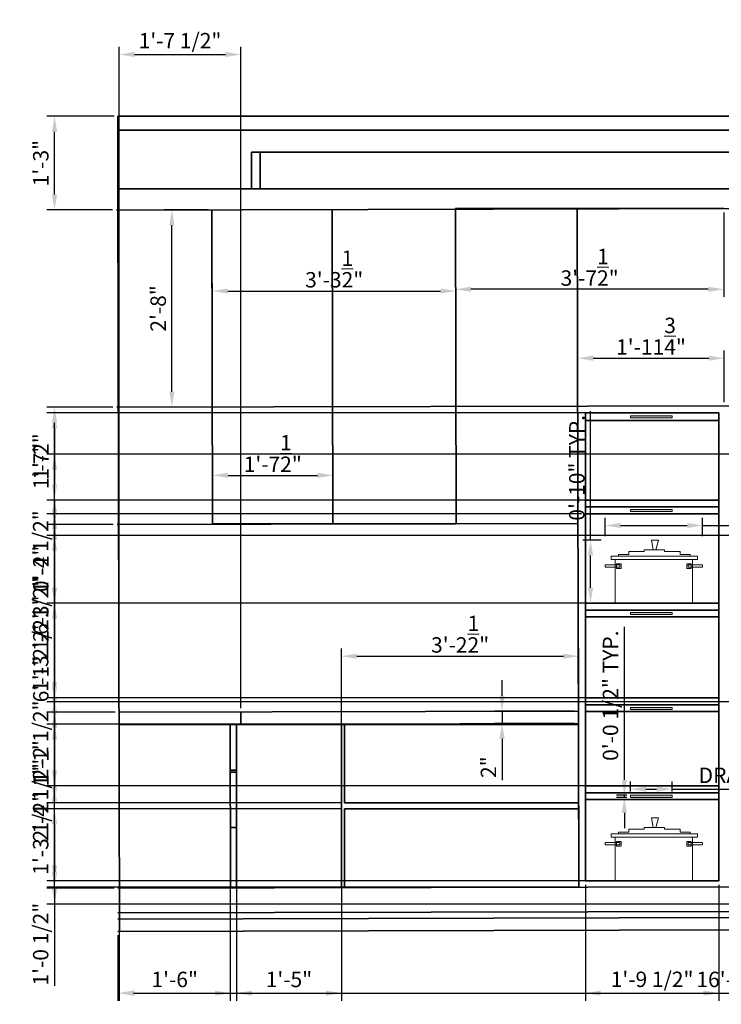
# Model space of a CAD drawing. Units: inches. Extents: x 1464 to 1689, y 996 to 1156.
# Tile 1 of 2: x 1464 to 1578, y 996 to 1156. Entities that reach past the tile are written whole.
import ezdxf

# ---------------------------------------------------------------- set-up
doc = ezdxf.new("R2010")
doc.units = ezdxf.units.IN
for name, color, linetype, lineweight in [('A-ANNO-DIMS', 2, 'Continuous', 18), ('A-ELEV', 7, 'Continuous', 35), ('A-EQPM', 9, 'Continuous', 18), ('A-FURN', 8, 'Continuous', 18)]:
    doc.layers.add(name, color=color, linetype=linetype, lineweight=lineweight)
doc.styles.get("Standard").update_dxf_attribs({"font": 'arial.ttf'})
doc.dimstyles.new('ISO-25', dxfattribs={"dimtxt": 2.5, "dimasz": 2.5, "dimexe": 1.25, "dimexo": 0.625, "dimtad": 1, "dimdec": 4, "dimlunit": 4, "dimtxsty": 'Standard', "dimcen": 2.5, "dimadec": 0, "dimazin": 0, "dimtfac": 1, "dimtdec": 4, "dimtmove": 0, "dimatfit": 3, "dimfxl": 1, "dimarcsym": 0})

# ---------------------------------------------------------------- blocks, each defined once
blk = doc.blocks.new('*D1')
at = {"layer": 'A-ANNO-DIMS', "color": 0, "lineweight": -2, "transparency": 16777216}
for p, q in [((1494.58, 1125.08), (1487.46, 1125.08)), ((1488.71, 1095.58), (1488.71, 1122.58)), ((1494.65, 1093.08), (1487.46, 1093.08))]:
    blk.add_line(p, q, dxfattribs=at)
at = {"layer": 'A-ANNO-DIMS', "color": 0, "transparency": 16777216}
for points in [[(1488.3, 1122.58), (1489.13, 1122.58), (1488.71, 1125.08)], [(1488.3, 1095.58), (1489.13, 1095.58), (1488.71, 1093.08)]]:
    blk.add_solid(points, dxfattribs=at)
at = {"layer": 'Defpoints', "color": 0, "transparency": 16777216}
for p in [(1488.71, 1125.08), (1495.21, 1125.08), (1495.28, 1093.08)]:
    blk.add_point(p, dxfattribs=at)
at = {"layer": 'A-ANNO-DIMS', "color": 0, "transparency": 16777216, "insert": (1486.81, 1109.08), "char_height": 2.5, "attachment_point": 5, "rotation": 90}
blk.add_mtext('2\'-8"', dxfattribs=at)
blk = doc.blocks.new('*D2')
at = {"layer": 'A-ANNO-DIMS', "color": 0, "lineweight": -2, "transparency": 16777216}
for p, q in [((1495.32, 1074.79), (1495.32, 1083.26)), ((1514.82, 1074.79), (1514.82, 1083.26)), ((1497.82, 1082.01), (1512.32, 1082.01))]:
    blk.add_line(p, q, dxfattribs=at)
at = {"layer": 'A-ANNO-DIMS', "color": 0, "transparency": 16777216}
for points in [[(1497.82, 1082.43), (1497.82, 1081.59), (1495.32, 1082.01)], [(1512.32, 1082.43), (1512.32, 1081.59), (1514.82, 1082.01)]]:
    blk.add_solid(points, dxfattribs=at)
at = {"layer": 'Defpoints', "color": 0, "transparency": 16777216}
for p in [(1514.82, 1082.01), (1495.32, 1074.17), (1514.82, 1074.17)]:
    blk.add_point(p, dxfattribs=at)
at = {"layer": 'A-ANNO-DIMS', "color": 0, "transparency": 16777216, "insert": (1505.07, 1085.56), "char_height": 2.5, "attachment_point": 5}
blk.add_mtext('1\'-7{\\H1x;\\S1/2;}"', dxfattribs=at)
blk = doc.blocks.new('*D3')
at = {"layer": 'A-ANNO-DIMS', "color": 0, "lineweight": -2, "transparency": 16777216}
for p, q in [((1534.7, 1124.64), (1534.7, 1110.94)), ((1578.2, 1124.64), (1578.2, 1110.94)), ((1575.7, 1112.19), (1537.2, 1112.19))]:
    blk.add_line(p, q, dxfattribs=at)
at = {"layer": 'A-ANNO-DIMS', "color": 0, "transparency": 16777216}
for points in [[(1537.2, 1112.6), (1537.2, 1111.77), (1534.7, 1112.19)], [(1575.7, 1112.6), (1575.7, 1111.77), (1578.2, 1112.19)]]:
    blk.add_solid(points, dxfattribs=at)
at = {"layer": 'Defpoints', "color": 0, "transparency": 16777216}
for p in [(1534.7, 1125.27), (1578.2, 1125.27), (1534.7, 1112.19)]:
    blk.add_point(p, dxfattribs=at)
at = {"layer": 'A-ANNO-DIMS', "color": 0, "transparency": 16777216, "insert": (1556.45, 1115.76), "char_height": 2.5, "attachment_point": 5}
blk.add_mtext('3\'-7{\\H1x;\\S1/2;}"', dxfattribs=at)
blk = doc.blocks.new('*D4')
at = {"layer": 'A-ANNO-DIMS', "color": 0, "lineweight": -2, "transparency": 16777216}
for p, q in [((1495.28, 1093.71), (1495.28, 1113.16)), ((1497.78, 1111.91), (1532.28, 1111.91)), ((1534.78, 1093.79), (1534.78, 1113.16))]:
    blk.add_line(p, q, dxfattribs=at)
at = {"layer": 'A-ANNO-DIMS', "color": 0, "transparency": 16777216}
for points in [[(1497.78, 1112.32), (1497.78, 1111.49), (1495.28, 1111.91)], [(1532.28, 1112.32), (1532.28, 1111.49), (1534.78, 1111.91)]]:
    blk.add_solid(points, dxfattribs=at)
at = {"layer": 'Defpoints', "color": 0, "transparency": 16777216}
for p in [(1534.78, 1111.91), (1495.28, 1093.08), (1534.78, 1093.17)]:
    blk.add_point(p, dxfattribs=at)
at = {"layer": 'A-ANNO-DIMS', "color": 0, "transparency": 16777216, "insert": (1515.03, 1115.48), "char_height": 2.5, "attachment_point": 5}
blk.add_mtext('3\'-3{\\H1x;\\S1/2;}"', dxfattribs=at)
blk = doc.blocks.new('*D6')
at = {"layer": 'A-ANNO-DIMS', "color": 0, "lineweight": -2, "transparency": 16777216}
for p, q in [((1516.2, 1015.84), (1516.2, 1053.92)), ((1518.7, 1052.67), (1552.2, 1052.67)), ((1554.7, 1015.84), (1554.7, 1053.92))]:
    blk.add_line(p, q, dxfattribs=at)
at = {"layer": 'A-ANNO-DIMS', "color": 0, "transparency": 16777216}
for points in [[(1518.7, 1053.09), (1518.7, 1052.26), (1516.2, 1052.67)], [(1552.2, 1053.09), (1552.2, 1052.26), (1554.7, 1052.67)]]:
    blk.add_solid(points, dxfattribs=at)
at = {"layer": 'Defpoints', "color": 0, "transparency": 16777216}
for p in [(1554.7, 1052.67), (1516.2, 1015.21), (1554.7, 1015.21)]:
    blk.add_point(p, dxfattribs=at)
at = {"layer": 'A-ANNO-DIMS', "color": 0, "transparency": 16777216, "insert": (1535.45, 1056.25), "char_height": 2.5, "attachment_point": 5}
blk.add_mtext('3\'-2{\\H1x;\\S1/2;}"', dxfattribs=at)
blk = doc.blocks.new('*D9')
at = {"layer": 'A-ANNO-DIMS', "color": 0, "lineweight": -2, "transparency": 16777216}
for p, q in [((1554.53, 1093.84), (1554.53, 1102.26)), ((1578.28, 1093.89), (1578.28, 1102.26)), ((1557.03, 1101.01), (1575.78, 1101.01))]:
    blk.add_line(p, q, dxfattribs=at)
at = {"layer": 'A-ANNO-DIMS', "color": 0, "transparency": 16777216}
for points in [[(1557.03, 1101.43), (1557.03, 1100.6), (1554.53, 1101.01)], [(1575.78, 1101.43), (1575.78, 1100.6), (1578.28, 1101.01)]]:
    blk.add_solid(points, dxfattribs=at)
at = {"layer": 'Defpoints', "color": 0, "transparency": 16777216}
for p in [(1578.28, 1101.01), (1554.53, 1093.21), (1578.28, 1093.27)]:
    blk.add_point(p, dxfattribs=at)
at = {"layer": 'A-ANNO-DIMS', "color": 0, "transparency": 16777216, "insert": (1566.4, 1104.58), "char_height": 2.5, "attachment_point": 5}
blk.add_mtext('1\'-11{\\H1x;\\S3/4;}"', dxfattribs=at)
blk = doc.blocks.new('*D13')
at = {"layer": 'A-ANNO-DIMS', "color": 0, "lineweight": -2, "transparency": 16777216}
for p, q in [((1542.25, 1046.26), (1542.25, 1048.76)), ((1554.02, 1043.76), (1541, 1043.76)), ((1542.25, 1043.76), (1542.25, 1041.76)), ((1554.02, 1041.76), (1541, 1041.76)), ((1542.25, 1039.26), (1542.25, 1032.59))]:
    blk.add_line(p, q, dxfattribs=at)
at = {"layer": 'A-ANNO-DIMS', "color": 0, "transparency": 16777216}
for points in [[(1541.83, 1046.26), (1542.67, 1046.26), (1542.25, 1043.76)], [(1541.83, 1039.26), (1542.67, 1039.26), (1542.25, 1041.76)]]:
    blk.add_solid(points, dxfattribs=at)
at = {"layer": 'Defpoints', "color": 0, "transparency": 16777216}
for p in [(1554.64, 1043.76), (1542.25, 1041.76), (1554.64, 1041.76)]:
    blk.add_point(p, dxfattribs=at)
at = {"layer": 'A-ANNO-DIMS', "color": 0, "transparency": 16777216, "insert": (1540.37, 1034.67), "char_height": 2.5, "attachment_point": 5, "rotation": 90}
blk.add_mtext('2"', dxfattribs=at)
blk = doc.blocks.new('DRAWER-PULL')
h = blk.add_hatch(color=256)
h.dxf.hatch_style = 1
h.paths.add_polyline_path([(1569.81, 1030.11), (1563.08, 1030.11), (1563.08, 1029.76), (1569.81, 1029.77)])
for p, q in [((1563.08, 1030.11), (1563.08, 1029.76)), ((1569.81, 1030.11), (1563.08, 1030.11)), ((1563.08, 1029.76), (1569.81, 1029.77)), ((1569.81, 1029.77), (1569.81, 1030.11))]:
    blk.add_line(p, q)
blk = doc.blocks.new('COOKING-POT')
for p, q in [((1566.51, 1026.47), (1567.6, 1026.47)), ((1566.51, 1026.47), (1566.73, 1024.87)), ((1567.6, 1026.47), (1567.2, 1024.87)), ((1559.93, 1023.33), (1559.93, 1023.87)), ((1559.93, 1023.87), (1573.97, 1023.87)), ((1559.93, 1023.87), (1561.16, 1023.87)), ((1573.97, 1023.87), (1559.93, 1023.87)), ((1561.16, 1023.87), (1561.16, 1024.13)), ((1561.16, 1024.13), (1562.79, 1024.13)), ((1562.79, 1024.13), (1562.79, 1024.63)), ((1562.79, 1024.63), (1565.31, 1024.63)), ((1565.31, 1024.63), (1565.31, 1024.87)), ((1565.31, 1024.87), (1566.95, 1024.87)), ((1565.31, 1024.63), (1565.31, 1024.63)), ((1568.6, 1024.87), (1566.95, 1024.87)), ((1568.6, 1024.63), (1568.6, 1024.87)), ((1571.12, 1024.63), (1568.6, 1024.63)), ((1568.6, 1024.63), (1568.6, 1024.63)), ((1571.12, 1024.13), (1571.12, 1024.63)), ((1572.75, 1024.13), (1571.12, 1024.13)), ((1572.75, 1023.87), (1572.75, 1024.13)), ((1573.97, 1023.87), (1572.75, 1023.87)), ((1573.97, 1023.87), (1573.97, 1023.33)), ((1573.97, 1023.33), (1573.97, 1023.87)), ((1558.97, 1022.08), (1558.97, 1022.48)), ((1559.01, 1022.48), (1561.33, 1022.48)), ((1560.59, 1023.33), (1559.93, 1023.33)), ((1560.59, 1016.23), (1560.59, 1023.33)), ((1560.59, 1023.33), (1573.15, 1023.33)), ((1560.81, 1021.84), (1560.81, 1022.64)), ((1560.81, 1022.64), (1561.55, 1022.64)), ((1561.33, 1022.48), (1561.33, 1022.08)), ((1561.55, 1022.64), (1561.55, 1021.84)), ((1572.93, 1022.64), (1572.19, 1022.64)), ((1572.19, 1022.64), (1572.19, 1021.84)), ((1574.72, 1022.48), (1572.41, 1022.48)), ((1572.41, 1022.48), (1572.41, 1022.08)), ((1572.93, 1021.84), (1572.93, 1022.64)), ((1573.15, 1023.33), (1573.15, 1016.23)), ((1573.97, 1023.33), (1573.15, 1023.33)), ((1573.15, 1016.23), (1573.15, 1023.33)), ((1574.77, 1022.08), (1574.77, 1022.48)), ((1561.33, 1022.08), (1558.97, 1022.08)), ((1561.55, 1021.84), (1560.81, 1021.84)), ((1572.19, 1021.84), (1572.93, 1021.84)), ((1572.41, 1022.08), (1574.77, 1022.08))]:
    blk.add_line(p, q)
blk = doc.blocks.new('*D16')
at = {"layer": 'A-ANNO-DIMS', "color": 0, "lineweight": -2, "transparency": 16777216}
for p, q in [((1563.08, 1030.73), (1563.08, 1032.37)), ((1569.81, 1030.73), (1569.81, 1032.37)), ((1565.58, 1031.12), (1567.31, 1031.12)), ((1569.81, 1031.12), (1620.69, 1031.12))]:
    blk.add_line(p, q, dxfattribs=at)
at = {"layer": 'A-ANNO-DIMS', "color": 0, "transparency": 16777216}
for points in [[(1565.58, 1031.53), (1565.58, 1030.7), (1563.08, 1031.12)], [(1567.31, 1031.53), (1567.31, 1030.7), (1569.81, 1031.12)]]:
    blk.add_solid(points, dxfattribs=at)
at = {"layer": 'Defpoints', "color": 0, "transparency": 16777216}
for p in [(1569.81, 1031.12), (1563.08, 1030.11), (1569.81, 1030.11)]:
    blk.add_point(p, dxfattribs=at)
at = {"layer": 'A-ANNO-DIMS', "color": 0, "transparency": 16777216, "insert": (1596.5, 1033.03), "char_height": 2.5, "attachment_point": 5}
blk.add_mtext('DRAWER PULL 0\'-6 1/2" TYP.', dxfattribs=at)
blk = doc.blocks.new('*D17')
at = {"layer": 'A-ANNO-DIMS', "color": 0, "lineweight": -2, "transparency": 16777216}
for p, q in [((1562.08, 1032.61), (1562.08, 1057.42)), ((1562.46, 1030.11), (1560.83, 1030.11)), ((1562.46, 1029.76), (1560.83, 1029.76)), ((1562.08, 1029.76), (1562.08, 1030.11)), ((1562.08, 1027.26), (1562.08, 1024.76))]:
    blk.add_line(p, q, dxfattribs=at)
at = {"layer": 'A-ANNO-DIMS', "color": 0, "transparency": 16777216}
for points in [[(1561.66, 1032.61), (1562.49, 1032.61), (1562.08, 1030.11)], [(1561.66, 1027.26), (1562.49, 1027.26), (1562.08, 1029.76)]]:
    blk.add_solid(points, dxfattribs=at)
at = {"layer": 'Defpoints', "color": 0, "transparency": 16777216}
for p in [(1562.08, 1030.11), (1563.08, 1030.11), (1563.08, 1029.76)]:
    blk.add_point(p, dxfattribs=at)
at = {"layer": 'A-ANNO-DIMS', "color": 0, "transparency": 16777216, "insert": (1560.16, 1046.27), "char_height": 2.5, "attachment_point": 5, "rotation": 90}
blk.add_mtext('0\'-0 1/2" TYP.', dxfattribs=at)
blk = doc.blocks.new('*D18')
at = {"layer": 'A-ANNO-DIMS', "color": 0, "lineweight": -2, "transparency": 16777216}
for p, q in [((1558.97, 1072.14), (1558.97, 1075.13)), ((1574.77, 1072.14), (1574.77, 1075.13)), ((1561.47, 1073.88), (1572.27, 1073.88)), ((1574.77, 1073.88), (1619.34, 1073.88))]:
    blk.add_line(p, q, dxfattribs=at)
at = {"layer": 'A-ANNO-DIMS', "color": 0, "transparency": 16777216}
for points in [[(1561.47, 1074.3), (1561.47, 1073.46), (1558.97, 1073.88)], [(1572.27, 1074.3), (1572.27, 1073.46), (1574.77, 1073.88)]]:
    blk.add_solid(points, dxfattribs=at)
at = {"layer": 'Defpoints', "color": 0, "transparency": 16777216}
for p in [(1574.77, 1073.88), (1558.97, 1071.51), (1574.77, 1071.51)]:
    blk.add_point(p, dxfattribs=at)
at = {"layer": 'A-ANNO-DIMS', "color": 0, "transparency": 16777216, "insert": (1598.3, 1075.8), "char_height": 2.5, "attachment_point": 5}
blk.add_mtext('COOKING POT 1\'-4" TYP.', dxfattribs=at)
blk = doc.blocks.new('*D19')
at = {"layer": 'A-ANNO-DIMS', "color": 0, "lineweight": -2, "transparency": 16777216}
for p, q in [((1556.6, 1071.51), (1556.6, 1092.44)), ((1558.34, 1071.51), (1555.35, 1071.51)), ((1556.6, 1063.77), (1556.6, 1069.01)), ((1558.34, 1061.27), (1555.35, 1061.27))]:
    blk.add_line(p, q, dxfattribs=at)
at = {"layer": 'A-ANNO-DIMS', "color": 0, "transparency": 16777216}
for points in [[(1556.18, 1069.01), (1557.02, 1069.01), (1556.6, 1071.51)], [(1556.18, 1063.77), (1557.02, 1063.77), (1556.6, 1061.27)]]:
    blk.add_solid(points, dxfattribs=at)
at = {"layer": 'Defpoints', "color": 0, "transparency": 16777216}
for p in [(1556.6, 1071.51), (1558.97, 1071.51), (1558.97, 1061.27)]:
    blk.add_point(p, dxfattribs=at)
at = {"layer": 'A-ANNO-DIMS', "color": 0, "transparency": 16777216, "insert": (1554.7, 1083.23), "char_height": 2.5, "attachment_point": 5, "rotation": 90}
blk.add_mtext('0\'-10" TYP.', dxfattribs=at)
blk = doc.blocks.new('*D20')
at = {"layer": 'A-ANNO-DIMS', "color": 0, "lineweight": -2, "transparency": 16777216}
for p, q in [((1676.97, 1007.86), (1676.97, 996.77)), ((1479.97, 1007.42), (1479.97, 996.77)), ((1482.47, 998.02), (1674.47, 998.02))]:
    blk.add_line(p, q, dxfattribs=at)
at = {"layer": 'A-ANNO-DIMS', "color": 0, "transparency": 16777216}
for points in [[(1482.47, 998.44), (1482.47, 997.6), (1479.97, 998.02)], [(1674.47, 998.44), (1674.47, 997.6), (1676.97, 998.02)]]:
    blk.add_solid(points, dxfattribs=at)
at = {"layer": 'Defpoints', "color": 0, "transparency": 16777216}
for p in [(1479.97, 1008.05), (1676.97, 1008.49), (1676.97, 998.02)]:
    blk.add_point(p, dxfattribs=at)
at = {"layer": 'A-ANNO-DIMS', "color": 0, "transparency": 16777216, "insert": (1578.47, 999.92), "char_height": 2.5, "attachment_point": 5}
blk.add_mtext('16\'-5"', dxfattribs=at)
blk = doc.blocks.new('*D22')
at = {"layer": 'A-ANNO-DIMS', "color": 0, "lineweight": -2, "transparency": 16777216}
for p, q in [((1479.53, 1043.59), (1468.43, 1043.59)), ((1469.68, 1017.55), (1469.68, 1041.09)), ((1479.33, 1015.05), (1468.43, 1015.05))]:
    blk.add_line(p, q, dxfattribs=at)
at = {"layer": 'A-ANNO-DIMS', "color": 0, "transparency": 16777216}
for points in [[(1469.26, 1041.09), (1470.1, 1041.09), (1469.68, 1043.59)], [(1469.26, 1017.55), (1470.1, 1017.55), (1469.68, 1015.05)]]:
    blk.add_solid(points, dxfattribs=at)
at = {"layer": 'Defpoints', "color": 0, "transparency": 16777216}
for p in [(1469.68, 1043.59), (1480.16, 1043.59), (1479.95, 1015.05)]:
    blk.add_point(p, dxfattribs=at)
at = {"layer": 'A-ANNO-DIMS', "color": 0, "transparency": 16777216, "insert": (1467.76, 1029.32), "char_height": 2.5, "attachment_point": 5, "rotation": 90}
blk.add_mtext('2\'-4 1/2"', dxfattribs=at)
blk = doc.blocks.new('*D23')
at = {"layer": 'A-ANNO-DIMS', "color": 0, "lineweight": -2, "transparency": 16777216}
for p, q in [((1479.19, 1074.05), (1468.43, 1074.05)), ((1469.68, 1046.09), (1469.68, 1071.55)), ((1479.53, 1043.59), (1468.43, 1043.59))]:
    blk.add_line(p, q, dxfattribs=at)
at = {"layer": 'A-ANNO-DIMS', "color": 0, "transparency": 16777216}
for points in [[(1469.26, 1071.55), (1470.1, 1071.55), (1469.68, 1074.05)], [(1469.26, 1046.09), (1470.1, 1046.09), (1469.68, 1043.59)]]:
    blk.add_solid(points, dxfattribs=at)
at = {"layer": 'Defpoints', "color": 0, "transparency": 16777216}
for p in [(1469.68, 1074.05), (1479.82, 1074.05), (1480.16, 1043.59)]:
    blk.add_point(p, dxfattribs=at)
at = {"layer": 'A-ANNO-DIMS', "color": 0, "transparency": 16777216, "insert": (1467.76, 1058.82), "char_height": 2.5, "attachment_point": 5, "rotation": 90}
blk.add_mtext('2\'-6 1/2"', dxfattribs=at)
blk = doc.blocks.new('*D24')
at = {"layer": 'A-ANNO-DIMS', "color": 0, "lineweight": -2, "transparency": 16777216}
for p, q in [((1479.15, 1093.05), (1468.43, 1093.05)), ((1469.68, 1076.55), (1469.68, 1090.55)), ((1479.19, 1074.05), (1468.43, 1074.05))]:
    blk.add_line(p, q, dxfattribs=at)
at = {"layer": 'A-ANNO-DIMS', "color": 0, "transparency": 16777216}
for points in [[(1469.26, 1090.55), (1470.1, 1090.55), (1469.68, 1093.05)], [(1469.26, 1076.55), (1470.1, 1076.55), (1469.68, 1074.05)]]:
    blk.add_solid(points, dxfattribs=at)
at = {"layer": 'Defpoints', "color": 0, "transparency": 16777216}
for p in [(1469.68, 1093.05), (1479.78, 1093.05), (1479.82, 1074.05)]:
    blk.add_point(p, dxfattribs=at)
at = {"layer": 'A-ANNO-DIMS', "color": 0, "transparency": 16777216, "insert": (1467.8, 1083.55), "char_height": 2.5, "attachment_point": 5, "rotation": 90}
blk.add_mtext('1\'-7"', dxfattribs=at)
blk = doc.blocks.new('*D25')
at = {"layer": 'A-ANNO-DIMS', "color": 0, "lineweight": -2, "transparency": 16777216}
for p, q in [((1479.34, 1140.25), (1468.43, 1140.25)), ((1469.68, 1127.55), (1469.68, 1137.75)), ((1479.08, 1125.05), (1468.43, 1125.05))]:
    blk.add_line(p, q, dxfattribs=at)
at = {"layer": 'A-ANNO-DIMS', "color": 0, "transparency": 16777216}
for points in [[(1469.26, 1137.75), (1470.1, 1137.75), (1469.68, 1140.25)], [(1469.26, 1127.55), (1470.1, 1127.55), (1469.68, 1125.05)]]:
    blk.add_solid(points, dxfattribs=at)
at = {"layer": 'Defpoints', "color": 0, "transparency": 16777216}
for p in [(1469.68, 1140.25), (1479.97, 1140.25), (1479.71, 1125.05)]:
    blk.add_point(p, dxfattribs=at)
at = {"layer": 'A-ANNO-DIMS', "color": 0, "transparency": 16777216, "insert": (1467.78, 1132.65), "char_height": 2.5, "attachment_point": 5, "rotation": 90}
blk.add_mtext('1\'-3"', dxfattribs=at)
blk = doc.blocks.new('*D27')
at = {"layer": 'A-ANNO-DIMS', "color": 0, "lineweight": -2, "transparency": 16777216}
for p, q in [((1632.43, 1085.44), (1468.43, 1085.44)), ((1469.68, 1014.98), (1469.68, 1082.94)), ((1632.43, 1012.48), (1468.43, 1012.48))]:
    blk.add_line(p, q, dxfattribs=at)
at = {"layer": 'A-ANNO-DIMS', "color": 0, "transparency": 16777216}
for points in [[(1469.26, 1082.94), (1470.1, 1082.94), (1469.68, 1085.44)], [(1469.26, 1014.98), (1470.1, 1014.98), (1469.68, 1012.48)]]:
    blk.add_solid(points, dxfattribs=at)
at = {"layer": 'Defpoints', "color": 0, "transparency": 16777216}
for p in [(1469.68, 1085.44), (1633.05, 1085.44), (1633.05, 1012.48)]:
    blk.add_point(p, dxfattribs=at)
at = {"layer": 'A-ANNO-DIMS', "color": 0, "transparency": 16777216, "insert": (1467.78, 1048.96), "char_height": 2.5, "attachment_point": 5, "rotation": 90}
blk.add_mtext('6\'-1"', dxfattribs=at)
blk = doc.blocks.new('*D29')
at = {"layer": 'A-ANNO-DIMS', "color": 0, "lineweight": -2, "transparency": 16777216}
for p, q in [((1480.16, 1044.22), (1480.16, 1151.52)), ((1499.9, 1044.26), (1499.9, 1151.52)), ((1482.66, 1150.27), (1497.4, 1150.27))]:
    blk.add_line(p, q, dxfattribs=at)
at = {"layer": 'A-ANNO-DIMS', "color": 0, "transparency": 16777216}
for points in [[(1482.66, 1150.69), (1482.66, 1149.86), (1480.16, 1150.27)], [(1497.4, 1150.69), (1497.4, 1149.86), (1499.9, 1150.27)]]:
    blk.add_solid(points, dxfattribs=at)
at = {"layer": 'Defpoints', "color": 0, "transparency": 16777216}
for p in [(1499.9, 1150.27), (1480.16, 1043.59), (1499.9, 1043.63)]:
    blk.add_point(p, dxfattribs=at)
at = {"layer": 'A-ANNO-DIMS', "color": 0, "transparency": 16777216, "insert": (1490.03, 1152.19), "char_height": 2.5, "attachment_point": 5}
blk.add_mtext('1\'-7 1/2"', dxfattribs=at)
blk = doc.blocks.new('*D30')
at = {"layer": 'A-ANNO-DIMS', "color": 0, "lineweight": -2, "transparency": 16777216}
for p, q in [((1480.16, 1040.97), (1480.16, 996.77)), ((1498.18, 1040.97), (1498.18, 996.77)), ((1482.66, 998.02), (1495.68, 998.02))]:
    blk.add_line(p, q, dxfattribs=at)
at = {"layer": 'A-ANNO-DIMS', "color": 0, "transparency": 16777216}
for points in [[(1482.66, 998.44), (1482.66, 997.6), (1480.16, 998.02)], [(1495.68, 998.44), (1495.68, 997.6), (1498.18, 998.02)]]:
    blk.add_solid(points, dxfattribs=at)
at = {"layer": 'Defpoints', "color": 0, "transparency": 16777216}
for p in [(1480.16, 1041.59), (1498.18, 1041.59), (1498.18, 998.02)]:
    blk.add_point(p, dxfattribs=at)
at = {"layer": 'A-ANNO-DIMS', "color": 0, "transparency": 16777216, "insert": (1489.17, 999.92), "char_height": 2.5, "attachment_point": 5}
blk.add_mtext('1\'-6"', dxfattribs=at)
blk = doc.blocks.new('*D31')
at = {"layer": 'A-ANNO-DIMS', "color": 0, "lineweight": -2, "transparency": 16777216}
for p, q in [((1499.18, 1040.97), (1499.18, 996.77)), ((1516.2, 1040.97), (1516.2, 996.77)), ((1501.68, 998.02), (1513.7, 998.02))]:
    blk.add_line(p, q, dxfattribs=at)
at = {"layer": 'A-ANNO-DIMS', "color": 0, "transparency": 16777216}
for points in [[(1501.68, 998.44), (1501.68, 997.6), (1499.18, 998.02)], [(1513.7, 998.44), (1513.7, 997.6), (1516.2, 998.02)]]:
    blk.add_solid(points, dxfattribs=at)
at = {"layer": 'Defpoints', "color": 0, "transparency": 16777216}
for p in [(1499.18, 1041.59), (1516.2, 1041.59), (1516.2, 998.02)]:
    blk.add_point(p, dxfattribs=at)
at = {"layer": 'A-ANNO-DIMS', "color": 0, "transparency": 16777216, "insert": (1507.69, 999.92), "char_height": 2.5, "attachment_point": 5}
blk.add_mtext('1\'-5"', dxfattribs=at)
blk = doc.blocks.new('*D32')
at = {"layer": 'A-ANNO-DIMS', "color": 0, "lineweight": -2, "transparency": 16777216}
for p, q in [((1516.08, 1041.67), (1468.43, 1041.67)), ((1469.68, 1039.17), (1469.68, 1031.4)), ((1516.08, 1028.9), (1468.43, 1028.9))]:
    blk.add_line(p, q, dxfattribs=at)
at = {"layer": 'A-ANNO-DIMS', "color": 0, "transparency": 16777216}
for points in [[(1469.26, 1039.17), (1470.1, 1039.17), (1469.68, 1041.67)], [(1469.26, 1031.4), (1470.1, 1031.4), (1469.68, 1028.9)]]:
    blk.add_solid(points, dxfattribs=at)
at = {"layer": 'Defpoints', "color": 0, "transparency": 16777216}
for p in [(1516.7, 1041.67), (1469.68, 1028.9), (1516.7, 1028.9)]:
    blk.add_point(p, dxfattribs=at)
at = {"layer": 'A-ANNO-DIMS', "color": 0, "transparency": 16777216, "insert": (1467.8, 1035.29), "char_height": 2.5, "attachment_point": 5, "rotation": 90}
blk.add_mtext('1\'-1"', dxfattribs=at)
blk = doc.blocks.new('*D33')
at = {"layer": 'A-ANNO-DIMS', "color": 0, "lineweight": -2, "transparency": 16777216}
for p, q in [((1516.08, 1027.9), (1468.43, 1027.9)), ((1469.68, 1025.4), (1469.68, 1017.71)), ((1516.08, 1015.21), (1468.43, 1015.21)), ((1469.68, 1015.21), (1469.68, 999.23))]:
    blk.add_line(p, q, dxfattribs=at)
at = {"layer": 'A-ANNO-DIMS', "color": 0, "transparency": 16777216}
for points in [[(1469.26, 1025.4), (1470.1, 1025.4), (1469.68, 1027.9)], [(1469.26, 1017.71), (1470.1, 1017.71), (1469.68, 1015.21)]]:
    blk.add_solid(points, dxfattribs=at)
at = {"layer": 'Defpoints', "color": 0, "transparency": 16777216}
for p in [(1516.7, 1027.9), (1469.68, 1015.21), (1516.7, 1015.21)]:
    blk.add_point(p, dxfattribs=at)
at = {"layer": 'A-ANNO-DIMS', "color": 0, "transparency": 16777216, "insert": (1467.76, 1005.97), "char_height": 2.5, "attachment_point": 5, "rotation": 90}
blk.add_mtext('1\'-0 1/2"', dxfattribs=at)
blk = doc.blocks.new('*D34')
at = {"layer": 'A-ANNO-DIMS', "color": 0, "lineweight": -2, "transparency": 16777216}
for p, q in [((1576.78, 1092.13), (1468.43, 1092.13)), ((1469.68, 1089.63), (1469.68, 1080.5)), ((1576.78, 1078), (1468.43, 1078))]:
    blk.add_line(p, q, dxfattribs=at)
at = {"layer": 'A-ANNO-DIMS', "color": 0, "transparency": 16777216}
for points in [[(1469.26, 1089.63), (1470.1, 1089.63), (1469.68, 1092.13)], [(1469.26, 1080.5), (1470.1, 1080.5), (1469.68, 1078)]]:
    blk.add_solid(points, dxfattribs=at)
at = {"layer": 'Defpoints', "color": 0, "transparency": 16777216}
for p in [(1577.4, 1092.13), (1469.68, 1078), (1577.4, 1078)]:
    blk.add_point(p, dxfattribs=at)
at = {"layer": 'A-ANNO-DIMS', "color": 0, "transparency": 16777216, "insert": (1467.8, 1085.07), "char_height": 2.5, "attachment_point": 5, "rotation": 90}
blk.add_mtext('1\'-2"', dxfattribs=at)
blk = doc.blocks.new('*D35')
at = {"layer": 'A-ANNO-DIMS', "color": 0, "lineweight": -2, "transparency": 16777216}
for p, q in [((1555.14, 1078), (1468.43, 1078)), ((1469.68, 1075.5), (1469.68, 1063.77)), ((1555.14, 1061.27), (1468.43, 1061.27))]:
    blk.add_line(p, q, dxfattribs=at)
at = {"layer": 'A-ANNO-DIMS', "color": 0, "transparency": 16777216}
for points in [[(1469.26, 1075.5), (1470.1, 1075.5), (1469.68, 1078)], [(1469.26, 1063.77), (1470.1, 1063.77), (1469.68, 1061.27)]]:
    blk.add_solid(points, dxfattribs=at)
at = {"layer": 'Defpoints', "color": 0, "transparency": 16777216}
for p in [(1555.76, 1078), (1469.68, 1061.27), (1555.76, 1061.27)]:
    blk.add_point(p, dxfattribs=at)
at = {"layer": 'A-ANNO-DIMS', "color": 0, "transparency": 16777216, "insert": (1467.76, 1069.63), "char_height": 2.5, "attachment_point": 5, "rotation": 90}
blk.add_mtext('1\'-4 1/2"', dxfattribs=at)
blk = doc.blocks.new('*D36')
at = {"layer": 'A-ANNO-DIMS', "color": 0, "lineweight": -2, "transparency": 16777216}
for p, q in [((1576.78, 1061.27), (1468.43, 1061.27)), ((1469.68, 1048.41), (1469.68, 1058.77)), ((1576.78, 1045.91), (1468.43, 1045.91))]:
    blk.add_line(p, q, dxfattribs=at)
at = {"layer": 'A-ANNO-DIMS', "color": 0, "transparency": 16777216}
for points in [[(1469.26, 1058.77), (1470.1, 1058.77), (1469.68, 1061.27)], [(1469.26, 1048.41), (1470.1, 1048.41), (1469.68, 1045.91)]]:
    blk.add_solid(points, dxfattribs=at)
at = {"layer": 'Defpoints', "color": 0, "transparency": 16777216}
for p in [(1469.68, 1061.27), (1577.4, 1061.27), (1577.4, 1045.91)]:
    blk.add_point(p, dxfattribs=at)
at = {"layer": 'A-ANNO-DIMS', "color": 0, "transparency": 16777216, "insert": (1467.76, 1053.59), "char_height": 2.5, "attachment_point": 5, "rotation": 90}
blk.add_mtext('1\'-3 1/2"', dxfattribs=at)
blk = doc.blocks.new('*D37')
at = {"layer": 'A-ANNO-DIMS', "color": 0, "lineweight": -2, "transparency": 16777216}
for p, q in [((1555.14, 1045.91), (1468.43, 1045.91)), ((1469.68, 1043.41), (1469.68, 1034.15)), ((1555.14, 1031.65), (1468.43, 1031.65))]:
    blk.add_line(p, q, dxfattribs=at)
at = {"layer": 'A-ANNO-DIMS', "color": 0, "transparency": 16777216}
for points in [[(1469.26, 1043.41), (1470.1, 1043.41), (1469.68, 1045.91)], [(1469.26, 1034.15), (1470.1, 1034.15), (1469.68, 1031.65)]]:
    blk.add_solid(points, dxfattribs=at)
at = {"layer": 'Defpoints', "color": 0, "transparency": 16777216}
for p in [(1555.76, 1045.91), (1469.68, 1031.65), (1555.76, 1031.65)]:
    blk.add_point(p, dxfattribs=at)
at = {"layer": 'A-ANNO-DIMS', "color": 0, "transparency": 16777216, "insert": (1467.76, 1038.78), "char_height": 2.5, "attachment_point": 5, "rotation": 90}
blk.add_mtext('1\'-2 1/2"', dxfattribs=at)
blk = doc.blocks.new('*D38')
at = {"layer": 'A-ANNO-DIMS', "color": 0, "lineweight": -2, "transparency": 16777216}
for p, q in [((1576.78, 1031.65), (1468.43, 1031.65)), ((1469.68, 1018.73), (1469.68, 1029.15)), ((1576.78, 1016.23), (1468.43, 1016.23))]:
    blk.add_line(p, q, dxfattribs=at)
at = {"layer": 'A-ANNO-DIMS', "color": 0, "transparency": 16777216}
for points in [[(1469.26, 1029.15), (1470.1, 1029.15), (1469.68, 1031.65)], [(1469.26, 1018.73), (1470.1, 1018.73), (1469.68, 1016.23)]]:
    blk.add_solid(points, dxfattribs=at)
at = {"layer": 'Defpoints', "color": 0, "transparency": 16777216}
for p in [(1469.68, 1031.65), (1577.4, 1031.65), (1577.4, 1016.23)]:
    blk.add_point(p, dxfattribs=at)
at = {"layer": 'A-ANNO-DIMS', "color": 0, "transparency": 16777216, "insert": (1467.76, 1023.94), "char_height": 2.5, "attachment_point": 5, "rotation": 90}
blk.add_mtext('1\'-3 1/2"', dxfattribs=at)
blk = doc.blocks.new('*D39')
at = {"layer": 'A-ANNO-DIMS', "color": 0, "lineweight": -2, "transparency": 16777216}
for p, q in [((1469.68, 1080.5), (1469.68, 1083)), ((1555.14, 1078), (1468.43, 1078)), ((1469.68, 1078), (1469.68, 1075.79)), ((1555.14, 1075.79), (1468.43, 1075.79)), ((1469.68, 1073.29), (1469.68, 1062.89))]:
    blk.add_line(p, q, dxfattribs=at)
at = {"layer": 'A-ANNO-DIMS', "color": 0, "transparency": 16777216}
for points in [[(1469.26, 1080.5), (1470.1, 1080.5), (1469.68, 1078)], [(1469.26, 1073.29), (1470.1, 1073.29), (1469.68, 1075.79)]]:
    blk.add_solid(points, dxfattribs=at)
at = {"layer": 'Defpoints', "color": 0, "transparency": 16777216}
for p in [(1555.76, 1078), (1469.68, 1075.79), (1555.76, 1075.79)]:
    blk.add_point(p, dxfattribs=at)
at = {"layer": 'A-ANNO-DIMS', "color": 0, "transparency": 16777216, "insert": (1467.78, 1066.84), "char_height": 2.5, "attachment_point": 5, "rotation": 90}
blk.add_mtext('0\'-2"', dxfattribs=at)
blk = doc.blocks.new('*D40')
at = {"layer": 'A-ANNO-DIMS', "color": 0, "lineweight": -2, "transparency": 16777216}
for p, q in [((1555.76, 1015.6), (1555.76, 996.77)), ((1577.4, 1015.6), (1577.4, 996.77)), ((1558.26, 998.02), (1574.9, 998.02))]:
    blk.add_line(p, q, dxfattribs=at)
at = {"layer": 'A-ANNO-DIMS', "color": 0, "transparency": 16777216}
for points in [[(1558.26, 998.44), (1558.26, 997.6), (1555.76, 998.02)], [(1574.9, 998.44), (1574.9, 997.6), (1577.4, 998.02)]]:
    blk.add_solid(points, dxfattribs=at)
at = {"layer": 'Defpoints', "color": 0, "transparency": 16777216}
for p in [(1555.76, 1016.23), (1577.4, 1016.23), (1577.4, 998.02)]:
    blk.add_point(p, dxfattribs=at)
at = {"layer": 'A-ANNO-DIMS', "color": 0, "transparency": 16777216, "insert": (1566.58, 999.94), "char_height": 2.5, "attachment_point": 5}
blk.add_mtext('1\'-9 1/2"', dxfattribs=at)
blk = doc.blocks.new('*D42')
at = {"layer": 'A-ANNO-DIMS', "color": 0, "lineweight": -2, "transparency": 16777216}
for p, q in [((1603.51, 1072.27), (1468.43, 1072.27)), ((1469.68, 1069.77), (1469.68, 1047.75)), ((1603.51, 1045.25), (1468.43, 1045.25))]:
    blk.add_line(p, q, dxfattribs=at)
at = {"layer": 'A-ANNO-DIMS', "color": 0, "transparency": 16777216}
for points in [[(1469.26, 1069.77), (1470.1, 1069.77), (1469.68, 1072.27)], [(1469.26, 1047.75), (1470.1, 1047.75), (1469.68, 1045.25)]]:
    blk.add_solid(points, dxfattribs=at)
at = {"layer": 'Defpoints', "color": 0, "transparency": 16777216}
for p in [(1604.13, 1072.27), (1469.68, 1045.25), (1604.13, 1045.25)]:
    blk.add_point(p, dxfattribs=at)
at = {"layer": 'A-ANNO-DIMS', "color": 0, "transparency": 16777216, "insert": (1467.78, 1058.76), "char_height": 2.5, "attachment_point": 5, "rotation": 90}
blk.add_mtext('2\'-3"', dxfattribs=at)

msp = doc.modelspace()

# ---------------------------------------------------------------- linework, layer by layer
at = {"layer": 'A-ELEV'}
for p, q in [((1479.96715, 1128.48751), (1479.96715, 1140.24723)), ((1479.96715, 1140.24723), (1676.96715, 1140.24723)), ((1676.96715, 1138.01467), (1479.96715, 1138.01467)), ((1501.63185, 1128.48751), (1501.63185, 1134.453)), ((1501.63185, 1134.453), (1666.33231, 1134.453)), ((1501.63185, 1134.453), (1501.63185, 1128.48751)), ((1503.02755, 1134.453), (1503.02755, 1128.48751)), ((1676.96715, 1128.48751), (1479.96715, 1128.48751)), ((1479.96715, 1128.48751), (1480.2373, 1008.04625)), ((1479.70522, 1125.04535), (1676.70473, 1125.48722)), ((1495.31958, 1074.16884), (1495.20539, 1125.08012)), ((1514.81958, 1074.16884), (1514.70529, 1125.12386)), ((1578.20497, 1125.26628), (1534.70497, 1125.26628)), ((1534.70497, 1125.26628), (1534.81958, 1074.16884)), ((1578.20497, 1125.26628), (1554.45497, 1125.26628)), ((1554.45497, 1125.26628), (1554.70182, 1015.21329)), ((1479.777, 1093.04543), (1676.7765, 1093.4873)), ((1555.76336, 1090.90808), (1577.4029, 1090.90808)), ((1555.76336, 1078.00137), (1577.4029, 1078.00137)), ((1555.76336, 1076.89088), (1577.4029, 1076.89088)), ((1555.76336, 1076.89088), (1577.4029, 1076.89088)), ((1555.76336, 1075.78925), (1577.4029, 1075.78925)), ((1555.76336, 1075.78038), (1577.4029, 1075.78038)), ((1479.81961, 1074.04548), (1554.56948, 1074.21314)), ((1534.81958, 1074.16884), (1495.31958, 1074.16884)), ((1495.31958, 1074.16884), (1514.81958, 1074.16884)), ((1567.50548, 1069.90699), (1567.50548, 1069.90699)), ((1555.76336, 1061.26841), (1577.4029, 1061.26841)), ((1555.76336, 1060.15791), (1577.4029, 1060.15791)), ((1555.76336, 1059.05628), (1577.4029, 1059.05628)), ((1555.76336, 1045.90981), (1577.4029, 1045.90981)), ((1555.76336, 1044.79931), (1577.4029, 1044.79931)), ((1554.64228, 1043.75761), (1480.15757, 1043.59055)), ((1480.15757, 1043.59055), (1480.15757, 1041.59055)), ((1499.8974, 1043.63482), (1499.8974, 1041.59055)), ((1554.64228, 1041.75761), (1554.64228, 1043.75761)), ((1555.76336, 1043.69768), (1577.4029, 1043.69768)), ((1480.15757, 1041.59055), (1516.20182, 1041.59055)), ((1498.21171, 1015.12976), (1498.1797, 1041.59055)), ((1498.1797, 1041.59055), (1554.64228, 1041.59055)), ((1499.21171, 1015.13097), (1499.1797, 1041.59175)), ((1516.20182, 1041.67139), (1554.64228, 1041.75761)), ((1516.20182, 1015.21329), (1516.20182, 1041.67139)), ((1516.70182, 1028.90192), (1516.70182, 1041.67139)), ((1554.64228, 1041.59055), (1554.70182, 1015.21329)), ((1498.18866, 1034.18603), (1499.18865, 1034.18724)), ((1498.18902, 1033.88624), (1499.18902, 1033.88745)), ((1555.76336, 1031.64825), (1577.4029, 1031.64825)), ((1555.76336, 1030.53775), (1577.4029, 1030.53775)), ((1554.67205, 1028.90192), (1516.70182, 1028.90192)), ((1555.76336, 1029.43612), (1577.4029, 1029.43612)), ((1516.70182, 1015.21329), (1516.70182, 1027.90192)), ((1554.67205, 1027.90192), (1516.70182, 1027.90192)), ((1498.19993, 1024.86843), (1499.19993, 1024.86964)), ((1567.50548, 1024.86818), (1567.50548, 1024.86818)), ((1479.95195, 1015.04563), (1625.70146, 1015.37254)), ((1480.2216, 1015.04623), (1516.20182, 1015.21329)), ((1554.70182, 1015.21329), (1516.20182, 1015.21329)), ((1479.96092, 1011.04564), (1676.96042, 1011.4875)), ((1479.96316, 1010.04564), (1676.96267, 1010.48751)), ((1479.96765, 1008.04565), (1676.96715, 1008.48751))]:
    msp.add_line(p, q, dxfattribs=at)
msp.add_lwpolyline([(1555.76336, 1092.13497), (1577.4029, 1092.13497), (1577.4029, 1016.22959), (1555.76336, 1016.22959)], close=True, dxfattribs=at)

# ---------------------------------------------------------------- block references
at = {"layer": 'A-EQPM'}
for p in [(0, 45.03881), (0, 0)]:
    msp.add_blockref('COOKING-POT', p, dxfattribs=at)
at = {"layer": 'A-FURN'}
for p in [(0, 61.5577), (0, 46.3589), (0, 29.66604), (0, 14.25103), (0, 0)]:
    msp.add_blockref('DRAWER-PULL', p, dxfattribs=at)

# ---------------------------------------------------------------- dimensions: what is measured, and where the dimension line sits
at = {"layer": 'A-ANNO-DIMS'}
for base, p1, p2, override, picture, middle in [((1499.8974, 1150.27223), (1480.15757, 1043.59055), (1499.8974, 1043.63482), {"dimdec": 1, "dimlfac": 1, "dimrnd": 0, "dimzin": 1, "dimdsep": 46, "dimlunit": 4, "dimfrac": 2}, '*D29', (1490.02749, 1152.18986)), ((1534.70497, 1112.18674), (1578.20497, 1125.26628), (1534.70497, 1125.26628), {"dimclrd": 0, "dimclre": 0, "dimclrt": 0}, '*D3', (1556.45497, 1115.76081)), ((1534.77697, 1111.90734), (1495.27717, 1093.0802), (1534.77697, 1093.1688), {"dimclrd": 0, "dimclre": 0, "dimclrt": 0}, '*D4', (1515.02707, 1115.48141)), ((1578.27675, 1101.014), (1554.52687, 1093.21309), (1578.27675, 1093.26636), {"dimclrd": 0, "dimclre": 0, "dimclrt": 0}, '*D9', (1566.40181, 1104.58295)), ((1514.81958, 1082.01144), (1495.31958, 1074.16884), (1514.81958, 1074.16884), {"dimclrd": 0, "dimclre": 0, "dimclrt": 0}, '*D2', (1505.06958, 1085.56334)), ((1554.70182, 1052.67435), (1516.20182, 1015.21329), (1554.70182, 1015.21329), {"dimclrd": 0, "dimclre": 0, "dimclrt": 0}, '*D6', (1535.45182, 1056.24841)), ((1498.1797, 998.02065), (1480.15757, 1041.59055), (1498.1797, 1041.59055), {"dimdec": 1, "dimlfac": 1, "dimrnd": 0, "dimzin": 1, "dimdsep": 46, "dimlunit": 4, "dimfrac": 2}, '*D30', (1489.16864, 999.92208)), ((1516.20182, 998.02065), (1499.1797, 1041.59175), (1516.20182, 1041.59055), {"dimdec": 1, "dimlfac": 1, "dimrnd": 0, "dimzin": 1, "dimdsep": 46, "dimlunit": 4, "dimfrac": 2}, '*D31', (1507.69076, 999.92208)), ((1577.4029, 998.02065), (1555.76336, 1016.22959), (1577.4029, 1016.22959), {"dimdec": 1, "dimlfac": 1, "dimrnd": 0, "dimzin": 1, "dimdsep": 46, "dimlunit": 4, "dimfrac": 2}, '*D40', (1566.58313, 999.93828)), ((1676.96715, 998.02065), (1479.96765, 1008.04565), (1676.96715, 1008.48751), {"dimdec": 1, "dimlfac": 1, "dimrnd": 0, "dimzin": 1, "dimdsep": 46, "dimlunit": 4, "dimfrac": 2}, '*D20', (1578.4674, 999.92208))]:
    dim = msp.add_linear_dim(base=base, p1=p1, p2=p2, dimstyle='ISO-25', override=override, dxfattribs=at)
    dim.commit()
    dim.dimension.update_dxf_attribs({"geometry": picture, "text_midpoint": middle})
for base, p1, p2, override, picture, middle in [((1469.68022, 1140.24723), (1479.70522, 1125.04535), (1479.96715, 1140.24723), {"dimdec": 1, "dimlfac": 1, "dimrnd": 0, "dimzin": 1, "dimdsep": 46, "dimlunit": 4, "dimfrac": 2}, '*D25', (1467.77794, 1132.64629)), ((1488.71187, 1125.08012), (1495.27717, 1093.0802), (1495.20539, 1125.08012), {"dimclrd": 0, "dimclre": 0, "dimclrt": 0}, '*D1', (1486.81044, 1109.08016)), ((1469.68022, 1093.04543), (1479.81961, 1074.04548), (1479.777, 1093.04543), {"dimdec": 1, "dimlfac": 1, "dimrnd": 0, "dimzin": 1, "dimdsep": 46, "dimlunit": 4, "dimfrac": 2}, '*D24', (1467.80011, 1083.54546)), ((1469.68022, 1078.00137), (1577.4029, 1092.13497), (1577.4029, 1078.00137), {"dimdec": 1, "dimlfac": 1, "dimrnd": 0, "dimzin": 1, "dimdsep": 46, "dimlunit": 4, "dimfrac": 2}, '*D34', (1467.80011, 1085.06817)), ((1469.68022, 1085.4387), (1633.05067, 1012.47552), (1633.05067, 1085.4387), {"dimdec": 1, "dimlfac": 1, "dimrnd": 0, "dimzin": 1, "dimdsep": 46, "dimlunit": 4, "dimfrac": 2}, '*D27', (1467.77879, 1048.95711)), ((1469.68022, 1075.78925), (1555.76336, 1078.00137), (1555.76336, 1075.78925), {"dimdec": 1, "dimlfac": 1, "dimrnd": 0, "dimzin": 1, "dimdsep": 46, "dimlunit": 4, "dimfrac": 2}, '*D39', (1467.77879, 1066.84143)), ((1469.68022, 1061.26841), (1555.76336, 1078.00137), (1555.76336, 1061.26841), {"dimdec": 1, "dimlfac": 1, "dimrnd": 0, "dimzin": 1, "dimdsep": 46, "dimlunit": 4, "dimfrac": 2}, '*D35', (1467.76259, 1069.63489)), ((1469.68022, 1074.04548), (1480.15757, 1043.59055), (1479.81961, 1074.04548), {"dimdec": 1, "dimlfac": 1, "dimrnd": 0, "dimzin": 1, "dimdsep": 46, "dimlunit": 4, "dimfrac": 2}, '*D23', (1467.76259, 1058.81801)), ((1469.68022, 1045.25324), (1604.13436, 1072.27429), (1604.13436, 1045.25324), {"dimdec": 1, "dimlfac": 1, "dimrnd": 0, "dimzin": 1, "dimdsep": 46, "dimlunit": 4, "dimfrac": 2}, '*D42', (1467.77794, 1058.76376)), ((1469.68022, 1061.26841), (1577.4029, 1045.90981), (1577.4029, 1061.26841), {"dimdec": 1, "dimlfac": 1, "dimrnd": 0, "dimzin": 1, "dimdsep": 46, "dimlunit": 4, "dimfrac": 2}, '*D36', (1467.76174, 1053.58911)), ((1542.2515, 1041.75761), (1554.64228, 1043.75761), (1554.64228, 1041.75761), {"dimclrd": 0, "dimclre": 0, "dimclrt": 0}, '*D13', (1540.37138, 1034.67456)), ((1469.68022, 1031.64825), (1555.76336, 1045.90981), (1555.76336, 1031.64825), {"dimdec": 1, "dimlfac": 1, "dimrnd": 0, "dimzin": 1, "dimdsep": 46, "dimlunit": 4, "dimfrac": 2}, '*D37', (1467.76259, 1038.77903)), ((1469.68022, 1043.59055), (1479.95195, 1015.04563), (1480.15757, 1043.59055), {"dimdec": 1, "dimlfac": 1, "dimrnd": 0, "dimzin": 1, "dimdsep": 46, "dimlunit": 4, "dimfrac": 2}, '*D22', (1467.76259, 1029.31809)), ((1469.68022, 1028.90192), (1516.70182, 1041.67139), (1516.70182, 1028.90192), {"dimdec": 1, "dimlfac": 1, "dimrnd": 0, "dimzin": 1, "dimdsep": 46, "dimlunit": 4, "dimfrac": 2}, '*D32', (1467.80011, 1035.28666)), ((1469.68022, 1031.64825), (1577.4029, 1016.22959), (1577.4029, 1031.64825), {"dimdec": 1, "dimlfac": 1, "dimrnd": 0, "dimzin": 1, "dimdsep": 46, "dimlunit": 4, "dimfrac": 2}, '*D38', (1467.76174, 1023.93892)), ((1469.68022, 1015.21329), (1516.70182, 1027.90192), (1516.70182, 1015.21329), {"dimdec": 1, "dimlfac": 1, "dimrnd": 0, "dimzin": 1, "dimdsep": 46, "dimlunit": 4, "dimfrac": 2}, '*D33', (1467.76259, 1005.97045))]:
    dim = msp.add_linear_dim(base=base, p1=p1, p2=p2, angle=90, dimstyle='ISO-25', override=override, dxfattribs=at)
    dim.commit()
    dim.dimension.update_dxf_attribs({"geometry": picture, "text_midpoint": middle})
for base, p1, p2, picture, middle in [((1556.59918, 1071.51053), (1558.96895, 1061.26841), (1558.96895, 1071.51053), '*D19', (1554.69775, 1083.22608)), ((1562.07591, 1030.10839), (1563.08417, 1029.76317), (1563.08417, 1030.10839), '*D17', (1560.15828, 1046.26545))]:
    dim = msp.add_linear_dim(base=base, p1=p1, p2=p2, angle=90, text='<> TYP.', dimstyle='ISO-25', override={"dimdec": 1, "dimlfac": 1, "dimrnd": 0, "dimzin": 1, "dimdsep": 46, "dimlunit": 4, "dimfrac": 2}, dxfattribs=at)
    dim.commit()
    dim.dimension.update_dxf_attribs({"geometry": picture, "text_midpoint": middle})
for base, p1, p2, text, picture, middle in [((1574.76738, 1073.8803), (1558.96895, 1071.51053), (1574.76738, 1071.51053), 'COOKING POT <> TYP.', '*D18', (1598.30421, 1075.79878)), ((1569.8059, 1031.11665), (1563.08417, 1030.10839), (1569.8059, 1030.10839), 'DRAWER PULL <> TYP.', '*D16', (1596.50013, 1033.03428))]:
    dim = msp.add_linear_dim(base=base, p1=p1, p2=p2, text=text, dimstyle='ISO-25', override={"dimdec": 1, "dimlfac": 1, "dimrnd": 0, "dimzin": 1, "dimdsep": 46, "dimlunit": 4, "dimfrac": 2}, dxfattribs=at)
    dim.commit()
    dim.dimension.update_dxf_attribs({"geometry": picture, "text_midpoint": middle})

doc.saveas('drawing.dxf')
